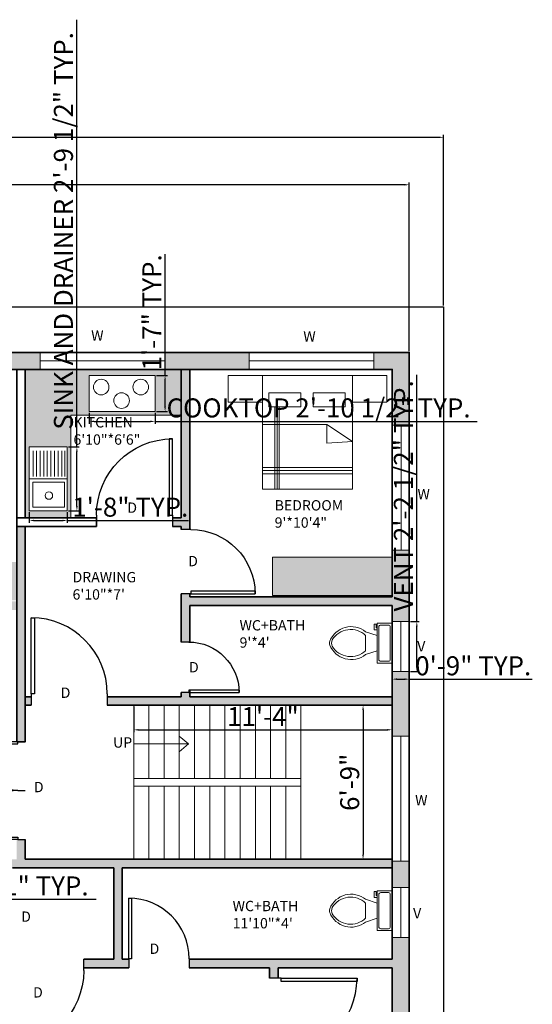
# Model space of a CAD drawing. Units: inches. Extents: x 2048 to 2702, y 2180 to 2964.
# Tile 3 of 3: x 2432 to 2702, y 2447 to 2964. Entities that reach past the tile are written whole.
import ezdxf

# ---------------------------------------------------------------- set-up
doc = ezdxf.new("R2010")
doc.units = ezdxf.units.IN
for name, color, linetype, lineweight in [('A-ANNO-DIMS', 2, 'Continuous', 13), ('A-ANNO-SYMB', 130, 'Continuous', 13), ('A-ANNO-TEXT', 130, 'Continuous', 18), ('A-AREA-IDEN', 130, 'Continuous', 18), ('A-CASE-PATT', 142, 'Continuous', 13), ('A-DOOR', 4, 'Continuous', 25), ('A-EQPM', 142, 'Continuous', 18), ('A-FLOR-FIXT', 142, 'Continuous', 18), ('A-FLOR-STRS', 7, 'Continuous', 18), ('A-FURN-PATT', 191, 'Continuous', 13), ('A-GLAZ', 4, 'Continuous', 18), ('A-WALL-PATT', 174, 'Continuous', 13), ('bed', 62, 'Continuous', 18), ('C-PROP', 7, 'Continuous', 25), ('kit', 142, 'Continuous', 18), ('TOI', 210, 'Continuous', 18), ('wall', 174, 'Continuous', 35), ('ward', 191, 'Continuous', 18)]:
    doc.layers.add(name, color=color, linetype=linetype, lineweight=lineweight)
doc.styles.get("Standard").update_dxf_attribs({"font": 'arial.ttf'})
doc.dimstyles.new('ISO-25', dxfattribs={"dimtxt": 10, "dimasz": 2.5, "dimexe": 1.25, "dimexo": 0.625, "dimtad": 1, "dimdec": 0, "dimlunit": 4, "dimtxsty": 'Standard', "dimcen": 2.5, "dimadec": 0, "dimazin": 0, "dimtfac": 1, "dimtdec": 0, "dimtmove": 0, "dimatfit": 3, "dimfxl": 1, "dimarcsym": 0})

# ---------------------------------------------------------------- blocks, each defined once
blk = doc.blocks.new('*U2')
for p, q in [((0, 0), (0, -6)), ((40, 0), (40, -6))]:
    blk.add_line(p, q)
blk.add_lwpolyline([(0, 0), (0, 40), (1.75, 40), (1.75, 0)], close=True)
blk.add_arc((0, 0), 40, 0, 90)
blk = doc.blocks.new('*U4')
for p, q in [((9.5, -6), (9.5, -2)), ((-10, -8.5), (-8, -8.5)), ((-10, -9.5), (-10, -8.5)), ((-7, -9.5), (-10, -9.5)), ((-8, -8.5), (-8, -8)), ((-7, -8), (-7, -9.5)), ((-4, -8), (-6, -14)), ((4, -8), (6, -14)), ((4, -14), (-4, -14))]:
    blk.add_line(p, q)
blk.add_lwpolyline([(10.5, -8), (10.5, 0), (-10.5, 0), (-10.5, -8)], close=True)
for points in [[(-9.5, -2), (-9.5, -6)], [(8.5, -1), (-8.5, -1)], [(-8.5, -7), (8.5, -7)]]:
    blk.add_lwpolyline(points)
for centre, radius, start, end in [((-8.62, -1.88), 0.884, 81.8699, 188.1301), ((8.62, -1.88), 0.884, 351.8699, 98.1301), ((-8.62, -6.12), 0.884, 171.8699, 278.1301), ((8.62, -6.12), 0.884, 261.8699, 8.1301), ((3.52, -21.58), 12.17, 141.4691, 247.9714), ((4.2, -21.82), 11.33, 136.3677, 238.9468), ((-3.52, -21.58), 12.17, 292.0284, 38.5307), ((-4.2, -21.82), 11.33, 301.053, 43.6321), ((0, -27.88), 4, 245.7318, 294.2682), ((0, -29), 4, 254.8605, 285.1395)]:
    blk.add_arc(centre, radius, start, end)
blk = doc.blocks.new('*D5')
at = {"layer": 'A-ANNO-DIMS', "color": 0, "lineweight": -2, "transparency": 16777216}
for p, q in [((2492.03, 2603.39), (2492.03, 2589.84)), ((2628.03, 2603.39), (2628.03, 2589.84)), ((2494.53, 2591.09), (2625.53, 2591.09))]:
    blk.add_line(p, q, dxfattribs=at)
at = {"layer": 'A-ANNO-DIMS', "color": 0, "transparency": 16777216}
for points in [[(2494.53, 2591.51), (2494.53, 2590.67), (2492.03, 2591.09)], [(2625.53, 2591.51), (2625.53, 2590.67), (2628.03, 2591.09)]]:
    blk.add_solid(points, dxfattribs=at)
at = {"layer": 'Defpoints', "color": 0, "transparency": 16777216}
for p in [(2492.03, 2604.01), (2628.03, 2604.01), (2628.03, 2591.09)]:
    blk.add_point(p, dxfattribs=at)
at = {"layer": 'A-ANNO-DIMS', "color": 0, "transparency": 16777216, "insert": (2560.03, 2596.74), "char_height": 10, "attachment_point": 5}
blk.add_mtext('11\'-4"', dxfattribs=at)
blk = doc.blocks.new('*D6')
at = {"layer": 'A-ANNO-DIMS', "color": 0, "lineweight": -2, "transparency": 16777216}
for p, q in [((2627.4, 2604.01), (2611.44, 2604.01)), ((2612.69, 2601.51), (2612.69, 2525.51)), ((2627.4, 2523.01), (2611.44, 2523.01))]:
    blk.add_line(p, q, dxfattribs=at)
at = {"layer": 'A-ANNO-DIMS', "color": 0, "transparency": 16777216}
for points in [[(2612.28, 2601.51), (2613.11, 2601.51), (2612.69, 2604.01)], [(2612.28, 2525.51), (2613.11, 2525.51), (2612.69, 2523.01)]]:
    blk.add_solid(points, dxfattribs=at)
at = {"layer": 'Defpoints', "color": 0, "transparency": 16777216}
for p in [(2628.03, 2604.01), (2612.69, 2523.01), (2628.03, 2523.01)]:
    blk.add_point(p, dxfattribs=at)
at = {"layer": 'A-ANNO-DIMS', "color": 0, "transparency": 16777216, "insert": (2606.96, 2563.51), "char_height": 10, "attachment_point": 5, "rotation": 90}
blk.add_mtext('6\'-9"', dxfattribs=at)
blk = doc.blocks.new('*D7')
at = {"layer": 'A-ANNO-DIMS', "color": 0, "lineweight": -2, "transparency": 16777216}
for p, q in [((2148.03, 2790.14), (2148.03, 2878.84)), ((2637.03, 2790.14), (2637.03, 2878.84)), ((2634.53, 2877.59), (2150.53, 2877.59))]:
    blk.add_line(p, q, dxfattribs=at)
at = {"layer": 'A-ANNO-DIMS', "color": 0, "transparency": 16777216}
for points in [[(2150.53, 2878), (2150.53, 2877.17), (2148.03, 2877.59)], [(2634.53, 2878), (2634.53, 2877.17), (2637.03, 2877.59)]]:
    blk.add_solid(points, dxfattribs=at)
at = {"layer": 'Defpoints', "color": 0, "transparency": 16777216}
for p in [(2148.03, 2877.59), (2148.03, 2789.51), (2637.03, 2789.51)]:
    blk.add_point(p, dxfattribs=at)
at = {"layer": 'A-ANNO-DIMS', "color": 0, "transparency": 16777216, "insert": (2392.53, 2883.32), "char_height": 10, "attachment_point": 5}
blk.add_mtext('40\'-9"', dxfattribs=at)
blk = doc.blocks.new('*D8')
at = {"layer": 'A-ANNO-DIMS', "color": 0, "lineweight": -2, "transparency": 16777216}
for p, q in [((2124.03, 2814.14), (2124.03, 2903.8)), ((2655.03, 2814.14), (2655.03, 2903.8)), ((2126.53, 2902.55), (2652.53, 2902.55))]:
    blk.add_line(p, q, dxfattribs=at)
at = {"layer": 'A-ANNO-DIMS', "color": 0, "transparency": 16777216}
for points in [[(2126.53, 2902.96), (2126.53, 2902.13), (2124.03, 2902.55)], [(2652.53, 2902.96), (2652.53, 2902.13), (2655.03, 2902.55)]]:
    blk.add_solid(points, dxfattribs=at)
at = {"layer": 'Defpoints', "color": 0, "transparency": 16777216}
for p in [(2655.03, 2902.55), (2124.03, 2813.51), (2655.03, 2813.51)]:
    blk.add_point(p, dxfattribs=at)
at = {"layer": 'A-ANNO-DIMS', "color": 0, "transparency": 16777216, "insert": (2389.53, 2908.28), "char_height": 10, "attachment_point": 5}
blk.add_mtext('44\'-3"', dxfattribs=at)
blk = doc.blocks.new('BED-DOUBLE-NIGHTSTANDS')
for p, q in [((24.5, 43.17), (24.5, 0)), ((25.71, 43.17), (25.71, 0)), ((26.92, 43.17), (26.92, 0)), ((18.01, 33.96), (51.87, 33.96)), ((51.87, 33.96), (65.5, 24.98)), ((51.87, 24.18), (51.87, 33.96)), ((65.5, 24.98), (51.87, 24.18)), ((18.01, 11.29), (65.5, 11.29)), ((18.01, 9.68), (65.5, 9.68)), ((18.01, 8.07), (65.5, 8.07))]:
    blk.add_line(p, q)
for points in [[(18.01, 59.74), (0, 59.74), (0, 45.7), (18.01, 45.7)], [(18.01, 59.74), (65.5, 59.74), (65.5, 0), (18.01, 0)], [(83.51, 59.74), (65.5, 59.74), (65.5, 45.7), (83.51, 45.7)], [(21.39, 50.51), (38.23, 50.51), (38.23, 43.17), (21.39, 43.17)], [(44.78, 50.51), (61.62, 50.51), (61.62, 43.17), (44.78, 43.17)]]:
    blk.add_lwpolyline(points, close=True)
blk = doc.blocks.new('COOKTOP-3-BURNER')
blk.add_lwpolyline([(0, 0), (34.65, 0), (34.65, 18.99), (0, 18.99)], close=True)
for centre in [(6.24, 12.85), (27.06, 12.85), (16.95, 5.75)]:
    blk.add_circle(centre, 4.1)
blk = doc.blocks.new('SINK-WITH-DRAINER')
for p, q in [((2.08, 18.11), (2.08, 31.52)), ((3.85, 18.11), (3.85, 31.52)), ((5.62, 18.11), (5.62, 31.52)), ((7.59, 18.11), (7.59, 31.52)), ((9.36, 18.11), (9.36, 31.52)), ((11.32, 18.11), (11.32, 31.52)), ((13.22, 18.11), (13.22, 31.52)), ((15.25, 18.11), (15.25, 31.52)), ((17.15, 18.11), (17.15, 31.52)), ((18.67, 18.11), (18.67, 31.52)), ((0, 16.82), (19.98, 16.82))]:
    blk.add_line(p, q)
for points in [[(0, 0), (19.98, 0), (19.98, 33.65), (0, 33.65)], [(1.93, 1.93), (18.53, 1.93), (18.53, 15.13), (1.93, 15.13)]]:
    blk.add_lwpolyline(points, close=True)
blk.add_circle((10.31, 8.05), 1.95)
blk = doc.blocks.new('WINDOW-WIDE')
blk.add_line((0, 4.49), (65.63, 4.49))
blk.add_lwpolyline([(0, 0), (65.63, 0), (65.63, 8.99), (0, 8.99)], close=True)
blk = doc.blocks.new('VENT-BATH')
blk.add_line((4.5, 26.32), (4.5, 0))
blk.add_lwpolyline([(0, 26.32), (9, 26.32), (9, 0), (0, 0)], close=True)
blk = doc.blocks.new('*D27')
at = {"layer": 'A-ANNO-DIMS', "color": 0, "lineweight": -2, "transparency": 16777216}
for p, q in [((2462.17, 2739.8), (2462.17, 2964.38)), ((2457.74, 2739.8), (2463.42, 2739.8)), ((2462.17, 2708.66), (2462.17, 2737.3)), ((2457.74, 2706.16), (2463.42, 2706.16))]:
    blk.add_line(p, q, dxfattribs=at)
at = {"layer": 'A-ANNO-DIMS', "color": 0, "transparency": 16777216}
for points in [[(2461.75, 2737.3), (2462.58, 2737.3), (2462.17, 2739.8)], [(2461.75, 2708.66), (2462.58, 2708.66), (2462.17, 2706.16)]]:
    blk.add_solid(points, dxfattribs=at)
at = {"layer": 'Defpoints', "color": 0, "transparency": 16777216}
for p in [(2457.12, 2739.8), (2462.17, 2739.8), (2457.12, 2706.16)]:
    blk.add_point(p, dxfattribs=at)
at = {"layer": 'A-ANNO-DIMS', "color": 0, "transparency": 16777216, "insert": (2456.37, 2853.34), "char_height": 10, "attachment_point": 5, "rotation": 90}
blk.add_mtext('SINK AND DRAINER 2\'-9 1/2" TYP.', dxfattribs=at)
blk = doc.blocks.new('*D28')
at = {"layer": 'A-ANNO-DIMS', "color": 0, "lineweight": -2, "transparency": 16777216}
for p, q in [((2437.14, 2705.53), (2437.14, 2699.86)), ((2457.12, 2705.53), (2457.12, 2699.86)), ((2439.64, 2701.11), (2454.62, 2701.11)), ((2457.12, 2701.11), (2520.88, 2701.11))]:
    blk.add_line(p, q, dxfattribs=at)
at = {"layer": 'A-ANNO-DIMS', "color": 0, "transparency": 16777216}
for points in [[(2439.64, 2701.53), (2439.64, 2700.69), (2437.14, 2701.11)], [(2454.62, 2701.53), (2454.62, 2700.69), (2457.12, 2701.11)]]:
    blk.add_solid(points, dxfattribs=at)
at = {"layer": 'Defpoints', "color": 0, "transparency": 16777216}
for p in [(2437.14, 2706.16), (2457.12, 2706.16), (2457.12, 2701.11)]:
    blk.add_point(p, dxfattribs=at)
at = {"layer": 'A-ANNO-DIMS', "color": 0, "transparency": 16777216, "insert": (2490.25, 2706.84), "char_height": 10, "attachment_point": 5}
blk.add_mtext('1\'-8" TYP.', dxfattribs=at)
blk = doc.blocks.new('*D29')
at = {"layer": 'A-ANNO-DIMS', "color": 0, "lineweight": -2, "transparency": 16777216}
for p, q in [((2468.7, 2757.78), (2468.7, 2751.96)), ((2503.35, 2757.78), (2503.35, 2751.96)), ((2471.2, 2753.21), (2500.85, 2753.21)), ((2503.35, 2753.21), (2672.75, 2753.21))]:
    blk.add_line(p, q, dxfattribs=at)
at = {"layer": 'A-ANNO-DIMS', "color": 0, "transparency": 16777216}
for points in [[(2471.2, 2753.63), (2471.2, 2752.79), (2468.7, 2753.21)], [(2500.85, 2753.63), (2500.85, 2752.79), (2503.35, 2753.21)]]:
    blk.add_solid(points, dxfattribs=at)
at = {"layer": 'Defpoints', "color": 0, "transparency": 16777216}
for p in [(2468.7, 2758.41), (2503.35, 2758.41), (2503.35, 2753.21)]:
    blk.add_point(p, dxfattribs=at)
at = {"layer": 'A-ANNO-DIMS', "color": 0, "transparency": 16777216, "insert": (2589.3, 2759.01), "char_height": 10, "attachment_point": 5}
blk.add_mtext('COOKTOP 2\'-10 1/2" TYP.', dxfattribs=at)
blk = doc.blocks.new('*D30')
at = {"layer": 'A-ANNO-DIMS', "color": 0, "lineweight": -2, "transparency": 16777216}
for p, q in [((2508.55, 2777.39), (2508.55, 2841.16)), ((2503.98, 2777.39), (2509.8, 2777.39)), ((2508.55, 2760.91), (2508.55, 2774.89)), ((2503.98, 2758.41), (2509.8, 2758.41))]:
    blk.add_line(p, q, dxfattribs=at)
at = {"layer": 'A-ANNO-DIMS', "color": 0, "transparency": 16777216}
for points in [[(2508.13, 2774.89), (2508.97, 2774.89), (2508.55, 2777.39)], [(2508.13, 2760.91), (2508.97, 2760.91), (2508.55, 2758.41)]]:
    blk.add_solid(points, dxfattribs=at)
at = {"layer": 'Defpoints', "color": 0, "transparency": 16777216}
for p in [(2503.35, 2777.39), (2508.55, 2777.39), (2503.35, 2758.41)]:
    blk.add_point(p, dxfattribs=at)
at = {"layer": 'A-ANNO-DIMS', "color": 0, "transparency": 16777216, "insert": (2502.9, 2810.53), "char_height": 10, "attachment_point": 5, "rotation": 90}
blk.add_mtext('1\'-7" TYP.', dxfattribs=at)
blk = doc.blocks.new('*D31')
at = {"layer": 'A-ANNO-DIMS', "color": 0, "lineweight": -2, "transparency": 16777216}
for p, q in [((2640.97, 2647.99), (2640.97, 2777.65)), ((2637.65, 2647.99), (2642.22, 2647.99)), ((2640.97, 2624.17), (2640.97, 2645.49)), ((2637.65, 2621.67), (2642.22, 2621.67))]:
    blk.add_line(p, q, dxfattribs=at)
at = {"layer": 'A-ANNO-DIMS', "color": 0, "transparency": 16777216}
for points in [[(2640.56, 2645.49), (2641.39, 2645.49), (2640.97, 2647.99)], [(2640.56, 2624.17), (2641.39, 2624.17), (2640.97, 2621.67)]]:
    blk.add_solid(points, dxfattribs=at)
at = {"layer": 'Defpoints', "color": 0, "transparency": 16777216}
for p in [(2637.03, 2647.99), (2640.97, 2647.99), (2637.03, 2621.67)]:
    blk.add_point(p, dxfattribs=at)
at = {"layer": 'A-ANNO-DIMS', "color": 0, "transparency": 16777216, "insert": (2635.18, 2714.07), "char_height": 10, "attachment_point": 5, "rotation": 90}
blk.add_mtext('VENT 2\'-2 1/2" TYP.', dxfattribs=at)
blk = doc.blocks.new('*D32')
at = {"layer": 'A-ANNO-DIMS', "color": 0, "lineweight": -2, "transparency": 16777216}
for p, q in [((2628.03, 2621.05), (2628.03, 2616.47)), ((2637.03, 2621.05), (2637.03, 2616.47)), ((2630.53, 2617.72), (2634.53, 2617.72)), ((2637.03, 2617.72), (2701.73, 2617.72))]:
    blk.add_line(p, q, dxfattribs=at)
at = {"layer": 'A-ANNO-DIMS', "color": 0, "transparency": 16777216}
for points in [[(2630.53, 2618.14), (2630.53, 2617.31), (2628.03, 2617.72)], [(2634.53, 2618.14), (2634.53, 2617.31), (2637.03, 2617.72)]]:
    blk.add_solid(points, dxfattribs=at)
at = {"layer": 'Defpoints', "color": 0, "transparency": 16777216}
for p in [(2628.03, 2621.67), (2637.03, 2621.67), (2637.03, 2617.72)]:
    blk.add_point(p, dxfattribs=at)
at = {"layer": 'A-ANNO-DIMS', "color": 0, "transparency": 16777216, "insert": (2670.63, 2623.45), "char_height": 10, "attachment_point": 5}
blk.add_mtext('0\'-9" TYP.', dxfattribs=at)
blk = doc.blocks.new('*D37')
at = {"layer": 'A-ANNO-DIMS', "color": 0, "lineweight": -2, "transparency": 16777216}
for p, q in [((2313.82, 2503.37), (2313.82, 2500.83)), ((2316.32, 2502.08), (2324.08, 2502.08)), ((2326.58, 2503.37), (2326.58, 2500.83)), ((2326.58, 2502.08), (2472.27, 2502.08))]:
    blk.add_line(p, q, dxfattribs=at)
at = {"layer": 'A-ANNO-DIMS', "color": 0, "transparency": 16777216}
for points in [[(2316.32, 2502.5), (2316.32, 2501.66), (2313.82, 2502.08)], [(2324.08, 2502.5), (2324.08, 2501.66), (2326.58, 2502.08)]]:
    blk.add_solid(points, dxfattribs=at)
at = {"layer": 'Defpoints', "color": 0, "transparency": 16777216}
for p in [(2313.82, 2503.99), (2326.58, 2503.99), (2326.58, 2502.08)]:
    blk.add_point(p, dxfattribs=at)
at = {"layer": 'A-ANNO-DIMS', "color": 0, "transparency": 16777216, "insert": (2400.67, 2507.73), "char_height": 10, "attachment_point": 5}
blk.add_mtext('END TABLE 1\'-1" TYP.', dxfattribs=at)

msp = doc.modelspace()

# ---------------------------------------------------------------- hatches: boundary and pattern name
at = {"layer": 'A-CASE-PATT'}
h = msp.add_hatch(color=256, dxfattribs=at)
h.dxf.hatch_style = 1
h.paths.add_polyline_path([(2264.28, 2565.56), (2181.03, 2565.56), (2181.03, 2601.56), (2157.03, 2601.56), (2157.03, 2541.56), (2264.28, 2541.56)])
h.paths.add_polyline_path([(2178.6, 2563.49), (2159.62, 2563.49), (2159.62, 2598.14), (2178.6, 2598.14)], flags=16)
h.paths.add_polyline_path([(2161.65, 2571.08, -1), (2169.85, 2571.08, -1)], flags=0)
h.paths.add_polyline_path([(2202.29, 2563.69), (2235.94, 2563.69), (2235.94, 2543.71), (2202.29, 2543.71)], flags=16)
h.paths.add_polyline_path([(2204.22, 2561.75), (2217.42, 2561.75), (2217.42, 2545.16), (2204.22, 2545.16)], flags=0)
h.paths.add_polyline_path([(2168.75, 2581.19, -1), (2176.95, 2581.19, -1)], flags=0)
h.paths.add_polyline_path([(2212.29, 2553.38, -1), (2208.39, 2553.38, -1)], flags=0)
h.paths.add_polyline_path([(2161.65, 2591.9, -1), (2169.85, 2591.9, -1)], flags=0)
h.paths.add_polyline_path([(2249.43, 2537.06), (2157.03, 2537.06), (2157.03, 2481.06), (2181.03, 2481.06), (2181.03, 2513.06), (2249.43, 2513.06)])
h.paths.add_polyline_path([(2178.15, 2520.97), (2178.15, 2486.32), (2159.16, 2486.32), (2159.16, 2520.97)], flags=16)
h.paths.add_polyline_path([(2201.45, 2534.49), (2235.1, 2534.49), (2235.1, 2514.51), (2201.45, 2514.51)], flags=16)
h.paths.add_polyline_path([(2203.38, 2532.56), (2216.58, 2532.56), (2216.58, 2515.96), (2203.38, 2515.96)], flags=0)
h.paths.add_polyline_path([(2169.4, 2514.73, -1), (2161.2, 2514.73, -1)], flags=0)
h.paths.add_polyline_path([(2176.5, 2504.02, -1), (2168.3, 2504.02, -1)], flags=0)
h.paths.add_polyline_path([(2211.45, 2524.18, -1), (2207.55, 2524.18, -1)], flags=0)
h.paths.add_polyline_path([(2169.4, 2493.91, -1), (2161.2, 2493.91, -1)], flags=0)
h.paths.add_polyline_path([(2628.03, 2372.19), (2627.36, 2372.19), (2627.36, 2424), (2604.03, 2424), (2604.03, 2365.01), (2568.03, 2365.01), (2568.03, 2341.01), (2628.03, 2341.01)])
h.paths.add_polyline_path([(2606.7, 2374.82), (2606.7, 2409.47), (2625.69, 2409.47), (2625.69, 2374.82)], flags=16)
h.paths.add_polyline_path([(2604.57, 2362.79), (2604.57, 2342.81), (2570.92, 2342.81), (2570.92, 2362.79)], flags=16)
h.paths.add_polyline_path([(2615.46, 2382.4, -1), (2623.66, 2382.4, -1)], flags=0)
h.paths.add_polyline_path([(2608.36, 2392.51, -1), (2616.56, 2392.51, -1)], flags=0)
h.paths.add_polyline_path([(2586.06, 2360.86), (2586.06, 2344.26), (2572.85, 2344.26), (2572.85, 2360.86)], flags=0)
h.paths.add_polyline_path([(2615.46, 2403.23, -1), (2623.66, 2403.23, -1)], flags=0)
h.paths.add_polyline_path([(2580.92, 2352.48, -1), (2577.03, 2352.48, -1)], flags=0)
h.paths.add_polyline_path([(2517.03, 2780.51), (2435.03, 2780.51), (2435.03, 2702.51), (2459.03, 2702.51), (2459.03, 2756.51), (2517.03, 2756.51)])
h.paths.add_polyline_path([(2468.7, 2777.39), (2503.35, 2777.39), (2503.35, 2758.41), (2468.7, 2758.41)], flags=16)
h.paths.add_polyline_path([(2470.84, 2771.26, -1), (2479.04, 2771.26, -1)], flags=0)
h.paths.add_polyline_path([(2457.12, 2739.8), (2457.12, 2706.16), (2437.14, 2706.16), (2437.14, 2739.8)], flags=16)
h.paths.add_polyline_path([(2489.75, 2764.16, -1), (2481.55, 2764.16, -1)], flags=0)
h.paths.add_polyline_path([(2491.66, 2771.26, -1), (2499.86, 2771.26, -1)], flags=0)
h.paths.add_polyline_path([(2455.67, 2721.29), (2455.67, 2708.09), (2439.07, 2708.09), (2439.07, 2721.29)], flags=0)
h.paths.add_polyline_path([(2449.4, 2714.21, -1), (2445.51, 2714.21, -1)], flags=0)
at = {"layer": 'A-FURN-PATT'}
h = msp.add_hatch(color=256, dxfattribs=at)
h.dxf.hatch_style = 1
h.paths.add_polyline_path([(2239.55, 2678.76), (2157.03, 2678.76), (2157.03, 2658.56), (2239.55, 2658.56)])
h.paths.add_polyline_path([(2430.53, 2679.37), (2367.61, 2679.37), (2367.61, 2659.17), (2430.53, 2659.17)])
h.paths.add_polyline_path([(2628.03, 2681.82), (2565.11, 2681.82), (2565.11, 2661.62), (2628.03, 2661.62)])
at = {"layer": 'A-WALL-PATT'}
h = msp.add_hatch(color=256, dxfattribs=at)
h.dxf.hatch_style = 1
h.paths.add_polyline_path([(2187.94, 2789.51), (2148.03, 2789.51), (2148.03, 2753.7), (2157.03, 2753.7), (2157.03, 2780.51), (2187.94, 2780.52)])
h.paths.add_polyline_path([(2337.86, 2789.51), (2253.56, 2789.51), (2253.56, 2780.55), (2306.03, 2780.56), (2310.53, 2780.56), (2310.53, 2780.56), (2337.86, 2780.56)])
h.paths.add_polyline_path([(2442.77, 2789.51), (2403.49, 2789.51), (2403.49, 2780.56), (2430.53, 2780.56), (2442.77, 2780.56)])
h.paths.add_polyline_path([(2157.03, 2678.76), (2157.03, 2688.07), (2148.03, 2688.07), (2148.03, 2645.92), (2157.03, 2645.92), (2157.03, 2658.56), (2157.03, 2658.56)])
h = msp.add_hatch(color=256, dxfattribs=at)
h.dxf.hatch_style = 1
h.paths.add_polyline_path([(2552.79, 2789.51), (2508.4, 2789.51), (2508.4, 2780.51), (2517.03, 2780.51), (2552.79, 2780.51)])
h.paths.add_polyline_path([(2637.03, 2789.51), (2618.42, 2789.51), (2618.42, 2780.51), (2628.03, 2780.51), (2628.03, 2751.2), (2637.03, 2751.2)])
h = msp.add_hatch(color=256, dxfattribs=at)
h.dxf.hatch_style = 1
h.paths.add_polyline_path([(2310.53, 2780.51), (2306.03, 2780.51), (2306.03, 2658.56), (2302.65, 2658.56), (2302.65, 2654.06), (2310.53, 2654.06), (2313.53, 2654.06), (2313.53, 2658.56), (2310.53, 2658.56)])
h.paths.add_polyline_path([(2262.65, 2658.56), (2157.03, 2658.56), (2157.03, 2654.06), (2255.03, 2654.06), (2262.65, 2654.06)])
h.paths.add_polyline_path([(2521.53, 2780.51), (2517.03, 2780.51), (2517.03, 2702.51), (2512.47, 2702.51), (2512.47, 2698.01), (2517.03, 2698.01), (2517.03, 2696.35), (2521.53, 2696.35), (2521.53, 2698.01)])
h.paths.add_polyline_path([(2628.03, 2608.51), (2521.53, 2608.51), (2521.53, 2610.77), (2521, 2610.77), (2517.03, 2610.77), (2517.03, 2608.51), (2487.03, 2608.51), (2478.14, 2608.51), (2478.14, 2604.01), (2487.03, 2604.01), (2592.01, 2604.01), (2628.03, 2604.01)])
h = msp.add_hatch(color=256, dxfattribs=at)
h.dxf.hatch_style = 1
h.paths.add_polyline_path([(2300.03, 2293.61), (2295.53, 2293.61), (2295.53, 2290.01), (2300.03, 2290.01)], flags=17)
h.paths.add_polyline_path([(2637.03, 2290.01), (2632.53, 2290.01), (2568.03, 2290.01), (2424.53, 2290.01), (2424.53, 2289.93), (2420.03, 2290.01), (2295.53, 2290.01), (2152.53, 2290.01), (2152.53, 2336.51), (2148.03, 2336.51), (2148.03, 2285.51), (2637.03, 2285.51)])
h.paths.add_polyline_path([(2424.53, 2465.93), (2420.03, 2466.01), (2420.03, 2290.01), (2424.53, 2289.93)])
h.paths.add_polyline_path([(2420.03, 2419.01), (2343.92, 2419.01), (2343.92, 2414.51), (2420.03, 2414.51)])
h.paths.add_polyline_path([(2637.03, 2522.1), (2628.03, 2522.1), (2628.03, 2508.22), (2637.03, 2508.22)])
h.paths.add_polyline_path([(2263.8, 2606.06), (2157.03, 2606.06), (2157.03, 2601.56), (2263.8, 2601.56)])
h.paths.add_polyline_path([(2259.53, 2626.68), (2255.69, 2626.68, -0.004462), (2255.23, 2626.68), (2255.03, 2626.68), (2255.03, 2606.07), (2259.53, 2606.06)])
h.paths.add_polyline_path([(2259.53, 2654.06), (2255.03, 2654.06), (2255.03, 2652.27), (2255.69, 2652.27), (2259.53, 2652.27)])
h.paths.add_polyline_path([(2310.53, 2606.06), (2306.03, 2606.06), (2306.03, 2518.51), (2310.53, 2518.51)])
h.paths.add_polyline_path([(2306.03, 2606.06), (2303.8, 2606.06), (2303.8, 2601.56), (2306.03, 2601.56)])
h.paths.add_polyline_path([(2306.03, 2541.56), (2157.03, 2541.56), (2157.03, 2537.06), (2306.03, 2537.06)])
h.paths.add_polyline_path([(2435.03, 2698.01), (2430.53, 2698.01), (2430.53, 2658.56), (2430.53, 2658.56), (2430.53, 2654.06), (2430.53, 2584.82), (2435.03, 2584.82)])
h.paths.add_polyline_path([(2430.53, 2658.56), (2353.53, 2658.56), (2353.53, 2654.06), (2430.53, 2654.06)])
h.paths.add_polyline_path([(2438.14, 2608.51), (2435.03, 2608.51), (2435.03, 2604.01), (2438.14, 2604.01)])
h = msp.add_hatch(color=256, dxfattribs=at)
h.dxf.hatch_style = 1
h.paths.add_polyline_path([(2637.03, 2621.67), (2628.03, 2621.67), (2628.03, 2608.51), (2628.03, 2587.75), (2637.03, 2587.75)])
h.paths.add_polyline_path([(2637.03, 2685.57), (2628.03, 2685.57), (2628.03, 2661.01), (2521.53, 2661.01), (2521.53, 2662.58), (2517.03, 2662.58), (2517.03, 2656.51), (2517.03, 2637.24), (2521, 2637.24, -0.005), (2521.53, 2637.24), (2521.53, 2656.51), (2628.03, 2656.51), (2628.03, 2647.99), (2637.03, 2647.99)])
h.paths.add_polyline_path([(2568.03, 2292.85), (2563.53, 2292.85), (2563.53, 2290.01), (2568.03, 2290.01)])
h = msp.add_hatch(color=256, dxfattribs=at)
h.dxf.hatch_style = 1
h.paths.add_polyline_path([(2157.03, 2554.63), (2148.03, 2554.63), (2148.03, 2525.8), (2157.03, 2525.8)])
h.paths.add_polyline_path([(2157.03, 2488.27), (2148.03, 2488.27), (2148.03, 2440.26), (2157.03, 2440.26)])
h.paths.add_polyline_path([(2168.96, 2345.51), (2157.03, 2345.51), (2157.03, 2374.63), (2148.03, 2374.63), (2148.03, 2336.51), (2152.53, 2336.51), (2168.96, 2336.51)])
h.paths.add_polyline_path([(2257.35, 2345.51), (2247.53, 2345.51), (2247.53, 2429.51), (2247.53, 2441.68), (2243.03, 2441.68), (2243.03, 2434.01), (2243.03, 2345.51), (2226.28, 2345.51), (2226.28, 2336.51), (2257.35, 2336.51)])
h.paths.add_polyline_path([(2300.03, 2414.51), (2303.92, 2414.51), (2303.92, 2419.01), (2300.03, 2419.01), (2300.03, 2434.01), (2277.86, 2434.01), (2277.86, 2429.51), (2295.53, 2429.51), (2295.53, 2409.26), (2295.53, 2345.51), (2283.92, 2345.51), (2283.92, 2336.51), (2295.53, 2336.51), (2295.53, 2327.38), (2300.03, 2327.38)])
h.paths.add_polyline_path([(2637.03, 2481.91), (2628.03, 2481.91), (2628.03, 2470.51), (2521.21, 2470.51), (2521.21, 2466.01), (2563.53, 2466.01), (2563.53, 2460.5), (2568.03, 2460.5), (2568.03, 2466.01), (2628.03, 2466.01), (2628.03, 2437.82), (2636.35, 2437.82), (2636.35, 2372.19), (2628.03, 2372.19), (2628.03, 2341.01), (2568.03, 2341.01), (2568.03, 2365.01), (2568.03, 2420.5), (2563.53, 2420.5), (2563.53, 2341.01), (2563.53, 2325.13), (2568.03, 2325.13), (2568.03, 2336.51), (2632.53, 2336.51), (2632.53, 2290.01), (2637.03, 2290.01)])
h.paths.add_polyline_path([(2263.16, 2481.06), (2162.03, 2481.06), (2157.03, 2481.06), (2157.03, 2476.56), (2205.4, 2476.56), (2263.16, 2476.56)])
h.paths.add_polyline_path([(2435.03, 2533.49), (2431.18, 2533.49), (2430.53, 2533.49), (2430.53, 2523.01), (2310.53, 2523.01), (2310.53, 2518.51), (2430.53, 2518.51), (2456.56, 2518.51), (2481.53, 2518.51), (2481.53, 2470.51), (2465.77, 2470.51), (2465.77, 2466.01), (2489.41, 2466.01), (2489.41, 2470.51), (2486.03, 2470.51), (2486.03, 2518.51), (2628.03, 2518.51), (2628.03, 2523.01), (2435.03, 2523.01)])
h.paths.add_polyline_path([(2310.53, 2518.51), (2306.03, 2518.51), (2306.03, 2481.06), (2303.16, 2481.06), (2303.16, 2476.56), (2310.53, 2476.56)])

# ---------------------------------------------------------------- linework, layer by layer
at = {"layer": 'A-ANNO-SYMB'}
for p, q in [((2492.03, 2583.67), (2520.89, 2583.67)), ((2520.89, 2583.67), (2516.03, 2587.79)), ((2520.89, 2583.67), (2516.03, 2579.55))]:
    msp.add_line(p, q, dxfattribs=at)
at = {"layer": 'A-FLOR-STRS'}
for p, q in [((2492.03, 2604.01), (2492.03, 2523.01)), ((2500.03, 2604.01), (2500.03, 2565.51)), ((2508.03, 2604.01), (2508.03, 2565.51)), ((2516.03, 2604.01), (2516.03, 2565.51)), ((2524.03, 2604.01), (2524.03, 2565.51)), ((2532.03, 2604.01), (2532.03, 2565.51)), ((2540.03, 2604.01), (2540.03, 2565.51)), ((2548.03, 2604.01), (2548.03, 2565.51)), ((2556.03, 2604.01), (2556.03, 2565.51)), ((2564.03, 2604.01), (2564.03, 2565.51)), ((2572.03, 2604.01), (2572.03, 2565.51)), ((2628.03, 2604.01), (2580.03, 2604.01)), ((2580.03, 2604.01), (2580.03, 2523.01)), ((2580.03, 2565.51), (2492.03, 2565.51)), ((2580.03, 2561.51), (2492.03, 2561.51)), ((2500.03, 2561.51), (2500.03, 2523.01)), ((2508.03, 2561.51), (2508.03, 2523.01)), ((2516.03, 2561.51), (2516.03, 2523.01)), ((2524.03, 2561.51), (2524.03, 2523.01)), ((2532.03, 2561.51), (2532.03, 2523.01)), ((2540.03, 2561.51), (2540.03, 2523.01)), ((2548.03, 2561.51), (2548.03, 2523.01)), ((2556.03, 2561.51), (2556.03, 2523.01)), ((2564.03, 2561.51), (2564.03, 2523.01)), ((2572.03, 2561.51), (2572.03, 2523.01))]:
    msp.add_line(p, q, dxfattribs=at)
at = {"layer": 'C-PROP'}
for p, q in [((2124.03, 2813.51), (2655.03, 2813.51)), ((2655.03, 2813.51), (2655.03, 2267.51))]:
    msp.add_line(p, q, dxfattribs=at)
at = {"layer": 'kit'}
for p, q in [((2517.03, 2780.51), (2517.03, 2756.51)), ((2459.03, 2702.51), (2459.03, 2756.51)), ((2517.03, 2756.51), (2459.03, 2756.51)), ((2435.03, 2702.51), (2459.03, 2702.51))]:
    msp.add_line(p, q, dxfattribs=at)
at = {"layer": 'wall'}
for p, q in [((2637.03, 2789.51), (2637.03, 2766.95)), ((2435.03, 2780.56), (2435.03, 2702.51)), ((2435.03, 2780.51), (2517.03, 2780.51)), ((2517.03, 2780.51), (2517.03, 2702.51)), ((2521.53, 2780.51), (2521.53, 2698.01)), ((2521.53, 2780.51), (2628.03, 2780.51)), ((2628.03, 2780.51), (2628.03, 2661.01)), ((2472.47, 2702.51), (2435.03, 2702.51)), ((2517.03, 2702.51), (2512.47, 2702.51)), ((2435.03, 2698.01), (2435.03, 2654.06)), ((2472.47, 2698.01), (2435.03, 2698.01)), ((2517.03, 2698.01), (2512.47, 2698.01)), ((2517.03, 2698.01), (2517.03, 2696.35)), ((2521.53, 2698.01), (2521.53, 2696.35)), ((2517.03, 2662.58), (2517.03, 2656.51)), ((2521.53, 2662.58), (2521.53, 2661.01)), ((2521.53, 2661.01), (2628.03, 2661.01)), ((2517.03, 2656.51), (2517.03, 2637.24)), ((2628.03, 2656.51), (2521.53, 2656.51)), ((2521.53, 2656.51), (2521.53, 2637.24)), ((2628.03, 2656.51), (2628.03, 2608.51)), ((2435.03, 2654.06), (2435.03, 2584.82)), ((2517.03, 2610.77), (2517.03, 2608.51)), ((2521.53, 2611.93), (2521.53, 2608.51)), ((2438.14, 2608.51), (2435.03, 2608.51)), ((2438.14, 2604.01), (2435.03, 2604.01)), ((2487.03, 2608.51), (2478.14, 2608.51)), ((2487.03, 2604.01), (2478.14, 2604.01)), ((2487.03, 2608.51), (2517.03, 2608.51)), ((2487.03, 2604.01), (2592.01, 2604.01)), ((2628.03, 2604.01), (2517.03, 2604.01)), ((2628.03, 2608.51), (2521.53, 2608.51)), ((2521.53, 2608.51), (2592.01, 2608.51)), ((2628.03, 2604.01), (2628.03, 2523.01)), ((2435.03, 2533.49), (2435.03, 2523.01)), ((2628.03, 2523.01), (2435.03, 2523.01)), ((2428.23, 2518.51), (2456.56, 2518.51)), ((2481.53, 2518.51), (2435.03, 2518.51)), ((2481.53, 2470.51), (2481.53, 2518.51)), ((2628.03, 2518.51), (2486.03, 2518.51)), ((2486.03, 2470.51), (2486.03, 2518.51)), ((2628.03, 2518.51), (2628.03, 2470.51)), ((2481.53, 2470.51), (2465.77, 2470.51)), ((2489.41, 2470.51), (2486.03, 2470.51)), ((2628.03, 2470.51), (2521.21, 2470.51)), ((2489.41, 2466.01), (2465.77, 2466.01)), ((2563.53, 2466.01), (2521.21, 2466.01)), ((2563.53, 2466.01), (2563.53, 2460.5)), ((2628.03, 2466.01), (2568.03, 2466.01)), ((2628.03, 2466.01), (2568.03, 2466.01)), ((2628.03, 2466.01), (2568.03, 2466.01)), ((2568.03, 2466.01), (2568.03, 2460.5))]:
    msp.add_line(p, q, dxfattribs=at)
for points in [[(2148.03, 2285.51), (2637.03, 2285.51), (2637.03, 2789.51), (2148.03, 2789.51)], [(2430.53, 2780.51), (2435.03, 2780.51), (2435.03, 2702.51), (2430.53, 2702.51)], [(2472.47, 2698.01), (2430.53, 2698.01), (2430.53, 2702.51), (2472.47, 2702.51)], [(2430.53, 2698.01), (2435.03, 2698.01), (2435.03, 2584.82), (2430.53, 2584.82)]]:
    msp.add_lwpolyline(points, close=True, dxfattribs=at)
for points in [[(2628.03, 2661.01), (2628.03, 2780.51), (2157.03, 2780.51), (2157.03, 2345.51)], [(2628.03, 2470.51), (2628.03, 2656.51)], [(2628.03, 2341.01), (2628.03, 2466.01)]]:
    msp.add_lwpolyline(points, dxfattribs=at)
at = {"layer": 'ward'}
msp.add_line((2565.11, 2661.62), (2565.11, 2681.82), dxfattribs=at)
msp.add_lwpolyline([(2565.11, 2661.62), (2628.03, 2661.62), (2628.03, 2681.82), (2565.11, 2681.82)], dxfattribs=at)

# ---------------------------------------------------------------- block references
at = {"layer": 'A-DOOR', "xscale": -1}
msp.add_blockref('*U2', (2512.47, 2704.01), dxfattribs=at)
at = {"layer": 'A-DOOR'}
for p, xscale, yscale, zscale, rotation in [((2522.09, 2662.58), -0.8441697781492633, 0.8441697781492633, 0.8441697781492633, 270), ((2521, 2610.77), -0.6617716164335441, 0.6617716164335441, 0.6617716164335441, 270), ((2431.18, 2584.82), -0.6417118160907794, 0.6417118160907794, 0.6417118160907794, 90), ((2431.18, 2533.49), 0.6417118160907794, 0.6417118160907794, 0.6417118160907794, 90)]:
    msp.add_blockref('*U2', p, dxfattribs=dict(at, xscale=xscale, yscale=yscale, zscale=zscale, rotation=rotation))
msp.add_blockref('*U2', (2438.14, 2610.01), dxfattribs=at)
at = {"layer": 'A-DOOR', "xscale": 0.7949714540024728, "yscale": 0.7949714540024728, "zscale": 0.7949714540024728}
msp.add_blockref('*U2', (2489.41, 2470.78), dxfattribs=at)
at = {"layer": 'A-DOOR', "xscale": -1, "rotation": 180}
msp.add_blockref('*U2', (2425.77, 2464.51), dxfattribs=at)
at = {"layer": 'A-DOOR', "rotation": 270}
msp.add_blockref('*U2', (2569.53, 2460.5), dxfattribs=at)
at = {"layer": 'A-EQPM'}
msp.add_blockref('COOKTOP-3-BURNER', (2468.7, 2758.41), dxfattribs=at)
at = {"layer": 'A-FLOR-FIXT'}
msp.add_blockref('SINK-WITH-DRAINER', (2437.14, 2706.16), dxfattribs=at)
at = {"layer": 'A-GLAZ'}
for name, p in [('WINDOW-WIDE', (2442.77, 2780.52)), ('WINDOW-WIDE', (2552.79, 2780.52)), ('VENT-BATH', (2628.03, 2621.67)), ('VENT-BATH', (2628.03, 2481.91))]:
    msp.add_blockref(name, p, dxfattribs=at)
for p, rotation in [((2628.2, 2751.2), 270), ((2628.03, 2587.75), 269.9999999999994)]:
    msp.add_blockref('WINDOW-WIDE', p, dxfattribs=dict(at, rotation=rotation))
at = {"layer": 'bed'}
msp.add_blockref('BED-DOUBLE-NIGHTSTANDS', (2541.72, 2717.66), dxfattribs=at)
at = {"layer": 'TOI', "rotation": 270}
for p in [(2628.03, 2636.68), (2628.03, 2496.02)]:
    msp.add_blockref('*U4', p, dxfattribs=at)

# ---------------------------------------------------------------- texts
at = {"layer": 'A-ANNO-TEXT', "attachment_point": 1}
for s, insert, char_height in [('W', (2469.68, 2801.04), 5.43), ('W', (2581.26, 2800.59), 5.43), ('W', (2641.33, 2717.75), 5.43), ('D', (2488.7, 2710.59), 5.43), ('D', (2520.71, 2682.49), 5.43), ('V', (2641.17, 2637.69), 5.43), ('D', (2521.15, 2626.72), 5.43), ('D', (2453.66, 2613.32), 5.43), ('UP', (2481.21, 2587.14), 5.433), ('D', (2439.55, 2563.72), 5.43), ('W', (2640.09, 2556.76), 5.43), ('D', (2432.86, 2495.61), 5.43), ('V', (2639.03, 2497.34), 5.43), ('D', (2500.41, 2478.74), 5.43), ('D', (2439.13, 2455.78), 5.43)]:
    msp.add_mtext_dynamic_manual_height_columns(s, width=134.4203, gutter_width=27.16, heights=[14.7], dxfattribs=dict(at, insert=insert, char_height=char_height))
at = {"layer": 'A-AREA-IDEN', "char_height": 5.433, "attachment_point": 1}
for s, heights, insert in [('KITCHEN\\P6\'10"*6\'6"', [0], (2460.37, 2755.45)), ('BEDROOM\\P9\'*10\'4"', [0], (2566.19, 2711.82)), ('DRAWING\\P6\'10"*7\'', [0], (2459.88, 2674.05)), ("WC+BATH\\P9'*4'", [0], (2547.73, 2648.75)), ('WC+BATH\\P11\'10"*4\'', [14.7], (2544.08, 2501.19))]:
    msp.add_mtext_dynamic_manual_height_columns(s, width=134.4203, gutter_width=27.16, heights=heights, dxfattribs=dict(at, insert=insert))

# ---------------------------------------------------------------- dimensions: what is measured, and where the dimension line sits
at = {"layer": 'A-ANNO-DIMS'}
for base, p1, p2, text, picture, middle in [((2462.17, 2739.8), (2457.12, 2706.16), (2457.12, 2739.8), 'SINK AND DRAINER <> TYP.', '*D27', (2456.37, 2853.34)), ((2508.55, 2777.39), (2503.35, 2758.41), (2503.35, 2777.39), '<> TYP.', '*D30', (2502.9, 2810.53)), ((2640.97, 2647.99), (2637.03, 2621.67), (2637.03, 2647.99), 'VENT <> TYP.', '*D31', (2635.18, 2714.07))]:
    dim = msp.add_linear_dim(base=base, p1=p1, p2=p2, angle=90, text=text, dimstyle='ISO-25', override={"dimdec": 1, "dimlfac": 1, "dimrnd": 0, "dimzin": 1, "dimdsep": 46, "dimlunit": 4, "dimfrac": 2}, dxfattribs=at)
    dim.commit()
    dim.dimension.update_dxf_attribs({"geometry": picture, "text_midpoint": middle})
for base, p1, p2, picture, middle in [((2655.03, 2902.55), (2124.03, 2813.51), (2655.03, 2813.51), '*D8', (2389.53, 2908.28)), ((2148.03, 2877.59), (2637.03, 2789.51), (2148.03, 2789.51), '*D7', (2392.53, 2883.32)), ((2628.03, 2591.09), (2492.03, 2604.01), (2628.03, 2604.01), '*D5', (2560.03, 2596.74))]:
    dim = msp.add_linear_dim(base=base, p1=p1, p2=p2, dimstyle='ISO-25', override={"dimclrd": 0, "dimclre": 0, "dimclrt": 0}, dxfattribs=at)
    dim.commit()
    dim.dimension.update_dxf_attribs({"geometry": picture, "text_midpoint": middle})
for base, p1, p2, text, picture, middle in [((2503.3524, 2753.2104), (2468.7022, 2758.4079), (2503.3524, 2758.4079), 'COOKTOP <> TYP.', '*D29', (2589.3015, 2759.0093)), ((2457.12, 2701.11), (2437.14, 2706.16), (2457.12, 2706.16), '<> TYP.', '*D28', (2490.25, 2706.84)), ((2637.03, 2617.72), (2628.03, 2621.67), (2637.03, 2621.67), '<> TYP.', '*D32', (2670.63, 2623.45)), ((2326.58, 2502.08), (2313.82, 2503.99), (2326.58, 2503.99), 'END TABLE <> TYP.', '*D37', (2400.67, 2507.73))]:
    dim = msp.add_linear_dim(base=base, p1=p1, p2=p2, text=text, dimstyle='ISO-25', override={"dimdec": 1, "dimlfac": 1, "dimrnd": 0, "dimzin": 1, "dimdsep": 46, "dimlunit": 4, "dimfrac": 2}, dxfattribs=at)
    dim.commit()
    dim.dimension.update_dxf_attribs({"geometry": picture, "text_midpoint": middle})
dim = msp.add_linear_dim(base=(2612.69, 2523.01), p1=(2628.03, 2604.01), p2=(2628.03, 2523.01), angle=90, dimstyle='ISO-25', override={"dimclrd": 0, "dimclre": 0, "dimclrt": 0}, dxfattribs=at)
dim.commit()
dim.dimension.update_dxf_attribs({"geometry": '*D6', "text_midpoint": (2606.96, 2563.51)})

doc.saveas('drawing.dxf')
